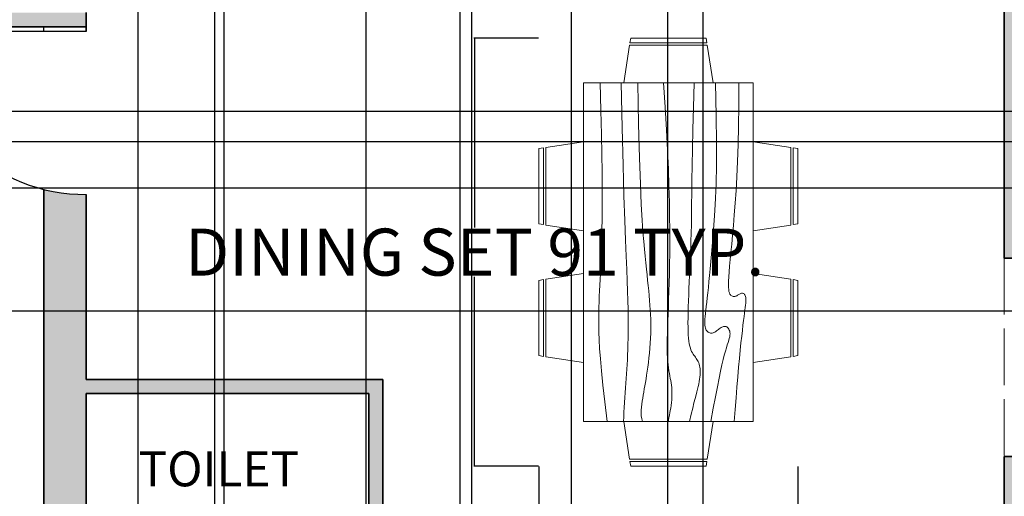
# Model space of a CAD drawing. Units: inches. Extents: x 300 to 1007, y 2 to 1069.
# Tile 3 of 12: x 557 to 766, y 170 to 271. Entities that reach past the tile are written whole.
import ezdxf

# ---------------------------------------------------------------- set-up
doc = ezdxf.new("R2010")
doc.units = ezdxf.units.IN
doc.header["$MEASUREMENT"] = 0
doc.linetypes.add('ACAD_ISO02W100', pattern=[15, 12, -3])
for name, color, linetype, lineweight in [('A-ANNO-DIMS', 2, 'Continuous', 18), ('A-AREA-IDEN', 7, 'Continuous', 18), ('A-DOOR', 3, 'Continuous', 25), ('A-FURN', 8, 'Continuous', 18), ('A-WALL', 7, 'Continuous', 35), ('A-WALL-OVHD', 8, 'ACAD_ISO02W100', 18)]:
    doc.layers.add(name, color=color, linetype=linetype, lineweight=lineweight)
doc.layers.add('A-WALL-PATT', color=9, linetype='Continuous', lineweight=9, true_color=0xc7c8ca)
doc.styles.get("Standard").update_dxf_attribs({"font": 'arial.ttf'})
doc.dimstyles.get("Standard").update_dxf_attribs({"dimtxt": 10, "dimasz": 0.18, "dimexe": 0.18, "dimexo": 0.0625, "dimgap": 0.09, "dimtad": 0, "dimtih": 1, "dimtoh": 1, "dimdec": 0, "dimzin": 0, "dimdsep": 46, "dimlunit": 3, "dimtxsty": 'Standard', "dimcen": 0.09, "dimadec": 0, "dimazin": 0, "dimtfac": 1, "dimtdec": 0, "dimtofl": 0, "dimtmove": 0, "dimatfit": 3, "dimfxl": 1, "dimtolj": 1, "dimtzin": 0, "dimarcsym": 0})

# ---------------------------------------------------------------- blocks, each defined once
blk = doc.blocks.new('Dining Set - 36 x 72 in.')
for p, q in [((-22, 27.5), (-22.1562, 26.50042)), ((-22, 27.5), (-6, 27.5)), ((-5.8437, 26.49966), (-6, 27.5)), ((6, 27.5), (5.8438, 26.50042)), ((6, 27.5), (22, 27.5)), ((22.1563, 26.49966), (22, 27.5)), ((-22.2343, 26.00059), (-23.4847, 17.99762)), ((-22.2304, 26), (-5.7608, 26)), ((-5.8416, 26.5), (-22.1534, 26.5)), ((-4.5152, 17.99762), (-5.7655, 25.99926)), ((5.7657, 26.00059), (4.5153, 17.99762)), ((5.7696, 26), (22.2392, 26)), ((22.1584, 26.5), (5.8466, 26.5)), ((23.4848, 17.99762), (22.2345, 25.99926)), ((36, 18), (-36, 18)), ((-36, 18), (-36, -18)), ((36, -18), (36, 18)), ((-44.0006, 8.23428), (-35.9976, 9.48474)), ((44.0006, 8.23428), (35.9976, 9.48474)), ((-45.5, 8), (-44.5004, 8.15617)), ((-45.5, 8), (-45.5, -8)), ((-44.5, -8.15843), (-44.5, 8.15338)), ((-44, 8.23041), (-44, -8.23915)), ((44, 8.23041), (44, -8.23915)), ((44.5, -8.15843), (44.5, 8.15338)), ((45.5, 8), (44.5005, 8.15617)), ((45.5, 8), (45.5, -8)), ((-44.4997, -8.15631), (-45.5, -8)), ((-35.9976, -9.48476), (-43.9993, -8.2345)), ((35.9976, -9.48476), (43.9993, -8.2345)), ((44.4997, -8.15631), (45.5, -8)), ((-36, -18), (36, -18)), ((-22.2343, -26.0006), (-23.4847, -17.99762)), ((-4.5152, -17.99762), (-5.7655, -25.99928)), ((5.7657, -26.0006), (4.5153, -17.99762)), ((23.4848, -17.99762), (22.2345, -25.99928)), ((-22.2304, -26), (-5.7608, -26)), ((-22, -27.5), (-22.1562, -26.50044)), ((-5.8416, -26.5), (-22.1534, -26.5)), ((-5.8437, -26.49967), (-6, -27.5)), ((5.7696, -26), (22.2392, -26)), ((6, -27.5), (5.8438, -26.50044)), ((22.1584, -26.5), (5.8466, -26.5)), ((22.1563, -26.49967), (22, -27.5)), ((-22, -27.5), (-6, -27.5)), ((6, -27.5), (22, -27.5))]:
    blk.add_line(p, q)
for points in [[(-36, 15), (-31.1772, 14.97754), (-26.8079, 14.91406), (-22.8538, 14.81543), (-19.276, 14.6875), (-16.0362, 14.53613), (-13.0957, 14.36718), (-10.4159, 14.18652), (-7.9583, 14), (-5.6904, 13.81315), (-3.6035, 13.63021), (-1.6954, 13.45508), (0.0365, 13.29166), (1.5945, 13.14388), (2.9811, 13.01562), (4.1988, 12.9108), (5.25, 12.83333), (6.1393, 12.78613), (6.8802, 12.76823), (7.4883, 12.77767), (7.9792, 12.8125), (8.3685, 12.87077), (8.6719, 12.95052), (8.9049, 13.0498), (9.0833, 13.16666), (9.2205, 13.29899), (9.3216, 13.44401), (9.3895, 13.59879), (9.4271, 13.76041), (9.4373, 13.92594), (9.4232, 14.09245), (9.3875, 14.257), (9.3333, 14.41666), (9.2638, 14.56917), (9.1836, 14.71484), (9.0975, 14.85465), (9.0104, 14.98958), (8.9272, 15.1206), (8.8529, 15.2487), (8.7922, 15.37483), (8.75, 15.5), (8.7305, 15.62467), (8.7344, 15.74739), (8.7617, 15.86621), (8.8125, 15.97916), (8.8867, 16.08431), (8.9844, 16.17968), (9.1055, 16.26334), (9.25, 16.33333), (9.4189, 16.38802), (9.6172, 16.42708), (9.8506, 16.45052), (10.125, 16.45833), (10.4463, 16.45052), (10.8203, 16.42708), (11.2529, 16.38802), (11.75, 16.33333), (12.3184, 16.26318), (12.9694, 16.17838), (13.7151, 16.07991), (14.5677, 15.96875), (15.5395, 15.84586), (16.6426, 15.71224), (17.8893, 15.56884), (19.2917, 15.41666), (20.859, 15.25667), (22.5879, 15.08984), (24.4721, 14.91715), (26.5052, 14.73958), (28.6809, 14.5581), (30.9929, 14.3737), (33.4347, 14.18733), (36, 14)], [(-36, 10), (-28.9766, 10.14274), (-23.1725, 10.20442), (-18.4241, 10.19775), (-14.5677, 10.13541), (-11.4399, 10.03011), (-8.877, 9.89453), (-6.7154, 9.74137), (-4.7917, 9.58333), (-2.9698, 9.43082), (-1.2246, 9.28515), (0.4415, 9.14534), (2.026, 9.01041), (3.5266, 8.87939), (4.9408, 8.7513), (6.266, 8.62516), (7.5, 8.5), (8.6411, 8.37549), (9.6914, 8.2539), (10.6538, 8.13818), (11.5312, 8.03125), (12.3267, 7.93603), (13.043, 7.85547), (13.6831, 7.79248), (14.25, 7.75), (14.7471, 7.7303), (15.1797, 7.73307), (15.5537, 7.75732), (15.875, 7.80208), (16.1494, 7.86637), (16.3828, 7.94922), (16.5811, 8.04964), (16.75, 8.16666), (16.8944, 8.29915), (17.0143, 8.44531), (17.1089, 8.60319), (17.1771, 8.77083), (17.218, 8.94629), (17.2305, 9.1276), (17.2137, 9.31282), (17.1667, 9.5), (17.0895, 9.6875), (16.987, 9.875), (16.8649, 10.0625), (16.7292, 10.25), (16.5856, 10.4375), (16.4401, 10.625), (16.2985, 10.8125), (16.1667, 11), (16.05, 11.18733), (15.9518, 11.3737), (15.8752, 11.5581), (15.8229, 11.73958), (15.798, 11.91715), (15.8034, 12.08984), (15.842, 12.25667), (15.9167, 12.41666), (16.0295, 12.56836), (16.1784, 12.70833), (16.3605, 12.83268), (16.5729, 12.9375), (16.8127, 13.01888), (17.0768, 13.07291), (17.3625, 13.0957), (17.6667, 13.08333), (17.9894, 13.03312), (18.3418, 12.94726), (18.7382, 12.82918), (19.1927, 12.68229), (19.7195, 12.51001), (20.3327, 12.31575), (21.0465, 12.10294), (21.875, 11.875), (22.8357, 11.63354), (23.959, 11.37304), (25.2786, 11.08618), (26.8282, 10.76562), (28.6414, 10.40405), (30.752, 9.99414), (33.1936, 9.52856), (36, 9)], [(-36, 5.5), (-30.7157, 5.3348), (-26.069, 5.20963), (-21.9946, 5.11767), (-18.4271, 5.05208), (-15.3009, 5.00602), (-12.5508, 4.97265), (-10.1112, 4.94515), (-7.9167, 4.91666), (-5.909, 4.88167), (-4.0586, 4.83984), (-2.3429, 4.79215), (-0.7396, 4.73958), (0.7739, 4.6831), (2.22, 4.6237), (3.6213, 4.56233), (5, 4.5), (6.373, 4.43782), (7.7344, 4.3776), (9.0723, 4.32129), (10.375, 4.27083), (11.6309, 4.22819), (12.8281, 4.19531), (13.9551, 4.17415), (15, 4.16666), (15.954, 4.17448), (16.819, 4.19791), (17.6001, 4.23698), (18.3021, 4.29166), (18.9299, 4.36198), (19.4883, 4.44791), (19.9823, 4.54948), (20.4167, 4.66666), (20.7969, 4.79899), (21.1302, 4.94401), (21.4245, 5.09879), (21.6875, 5.26041), (21.9271, 5.42594), (22.1511, 5.59245), (22.3672, 5.757), (22.5834, 5.91666), (22.8065, 6.06868), (23.0404, 6.21093), (23.2879, 6.34147), (23.5521, 6.45833), (23.8358, 6.55957), (24.142, 6.64323), (24.4735, 6.70735), (24.8334, 6.75), (25.2235, 6.76969), (25.642, 6.76692), (26.0858, 6.74267), (26.5521, 6.69791), (27.0379, 6.63362), (27.5404, 6.55078), (28.0565, 6.45036), (28.5834, 6.33333), (29.1242, 6.19987), (29.7071, 6.04687), (30.3661, 5.87044), (31.1354, 5.66666), (32.0493, 5.43164), (33.142, 5.16146), (34.4475, 4.85221), (36, 4.5)], [(-36, -1), (-30.7915, -0.6591), (-26.0195, -0.38216), (-21.6519, -0.16284), (-17.6563, 0.00521), (-14.0005, 0.12833), (-10.6523, 0.21289), (-7.5796, 0.26522), (-4.75, 0.29166), (-2.134, 0.29793), (0.2878, 0.28711), (2.5317, 0.26163), (4.6146, 0.22396), (6.5529, 0.17651), (8.3633, 0.12174), (10.0623, 0.06209), (11.6667, 0), (13.1899, -0.06201), (14.6341, -0.1211), (15.9982, -0.17432), (17.2813, -0.21875), (18.4823, -0.25147), (19.6003, -0.26953), (20.6343, -0.27002), (21.5834, -0.25), (22.4481, -0.20768), (23.2357, -0.14584), (23.9549, -0.06836), (24.6146, 0.02083), (25.2235, 0.11784), (25.7904, 0.21875), (26.3241, 0.31966), (26.8334, 0.41666), (27.3265, 0.50618), (27.8099, 0.58593), (28.2894, 0.65397), (28.7709, 0.70833), (29.2601, 0.74707), (29.763, 0.76823), (30.2855, 0.76985), (30.8334, 0.75), (31.4088, 0.70784), (31.9994, 0.64713), (32.589, 0.57275), (33.1615, 0.48958), (33.7008, 0.4025), (34.1908, 0.3164), (34.6153, 0.23616), (34.9584, 0.16666), (35.2099, 0.11165), (35.3848, 0.07031), (35.504, 0.04069), (35.5886, 0.02083), (35.6594, 0.00879), (35.7377, 0.0026), (35.8442, 0.00032), (36, 0)], [(-36, -6.5), (-27.1843, -6.31267), (-20.084, -6.1263), (-14.469, -5.9419), (-10.1094, -5.76042), (-6.7752, -5.58285), (-4.2363, -5.41016), (-2.2629, -5.24333), (-0.625, -5.08334), (0.8708, -4.93099), (2.2715, -4.78646), (3.5872, -4.64974), (4.8281, -4.52084), (6.0046, -4.39974), (7.127, -4.28646), (8.2053, -4.18099), (9.25, -4.08334), (10.2705, -3.99382), (11.2734, -3.91407), (12.2647, -3.84603), (13.25, -3.79167), (14.2354, -3.75293), (15.2266, -3.73177), (16.2295, -3.73015), (17.25, -3.75), (18.2912, -3.79248), (19.3451, -3.85547), (20.4009, -3.93604), (21.4479, -4.03125), (22.4754, -4.13819), (23.4727, -4.25391), (24.4289, -4.37549), (25.3334, -4.5), (26.1785, -4.62492), (26.9694, -4.74935), (27.7145, -4.87281), (28.4219, -4.99479), (29.1, -5.11483), (29.7572, -5.23242), (30.4016, -5.34709), (31.0417, -5.45834), (31.6837, -5.56437), (32.3262, -5.65821), (32.9658, -5.73153), (33.599, -5.77604), (34.2224, -5.78345), (34.8327, -5.74545), (35.4264, -5.65373), (36, -5.5)], [(-36, -10), (-26.4022, -9.81299), (-18.4675, -9.62891), (-11.9839, -9.45069), (-6.7396, -9.28125), (-2.5226, -9.12354), (0.8789, -8.98047), (3.6769, -8.85498), (6.0833, -8.75), (8.2767, -8.66765), (10.3021, -8.60677), (12.1712, -8.56543), (13.8958, -8.54167), (15.4876, -8.53353), (16.9583, -8.53907), (18.3197, -8.55632), (19.5834, -8.58334), (20.7616, -8.61841), (21.8685, -8.66081), (22.9188, -8.71004), (23.9271, -8.76563), (24.9081, -8.82707), (25.8763, -8.89388), (26.8465, -8.96558), (27.8334, -9.04167), (28.8474, -9.12118), (29.8828, -9.20117), (30.93, -9.27824), (31.9792, -9.34896), (33.0205, -9.40991), (34.0443, -9.45768), (35.0407, -9.48885), (36, -9.5)], [(-36, -14.5), (-30.0881, -14.33513), (-25.0332, -14.21224), (-20.7312, -14.12647), (-17.0781, -14.07292), (-13.97, -14.04671), (-11.3027, -14.04297), (-8.9724, -14.05681), (-6.875, -14.08334), (-4.9224, -14.11833), (-3.0905, -14.16016), (-1.3709, -14.20785), (0.2448, -14.26042), (1.7647, -14.3169), (3.1973, -14.3763), (4.5507, -14.43767), (5.8333, -14.5), (7.0554, -14.5621), (8.235, -14.62175), (9.3922, -14.67652), (10.5469, -14.72396), (11.7192, -14.76164), (12.929, -14.78711), (14.1965, -14.79794), (15.5417, -14.79167), (16.9933, -14.76424), (18.6152, -14.70508), (20.4804, -14.60197), (22.6615, -14.44271), (25.2312, -14.21509), (28.2624, -13.9069), (31.8277, -13.50594), (36, -13)]]:
    blk.add_lwpolyline(points)
blk = doc.blocks.new('DOOR-SINGLE-36')
for p, q in [((-1, 0), (-1, 36)), ((0, 0), (0, 36))]:
    blk.add_line(p, q)
blk.add_arc((0, 0.34), 35.66, 90, 180.5503)
blk = doc.blocks.new('*D53')
at = {"layer": 'A-ANNO-DIMS', "color": 0, "lineweight": -2, "transparency": 16777216}
for p, q in [((667.21, 266.96), (653.44, 266.96)), ((653.62, 266.78), (653.62, 226.72)), ((653.62, 176.14), (653.62, 216.2)), ((667.21, 175.96), (653.44, 175.96))]:
    blk.add_line(p, q, dxfattribs=at)
at = {"layer": 'A-ANNO-DIMS', "color": 0, "transparency": 16777216}
for points in [[(653.59, 266.78), (653.65, 266.78), (653.62, 266.96)], [(653.59, 176.14), (653.65, 176.14), (653.62, 175.96)]]:
    blk.add_solid(points, dxfattribs=at)
at = {"layer": 'Defpoints', "color": 0, "transparency": 16777216}
for p in [(667.27, 266.96), (653.62, 175.96), (667.27, 175.96)]:
    blk.add_point(p, dxfattribs=at)
at = {"layer": 'A-ANNO-DIMS', "color": 0, "transparency": 16777216, "insert": (653.62, 221.46), "char_height": 10, "attachment_point": 5}
blk.add_mtext('\\A1;DINING SET 91 TYP.', dxfattribs=at)
blk = doc.blocks.new('*D54')
at = {"layer": 'A-ANNO-DIMS', "color": 0, "lineweight": -2, "transparency": 16777216}
for p, q in [((667.27, 175.9), (667.27, 162.13)), ((722.27, 175.9), (722.27, 162.13)), ((667.45, 162.31), (670.34, 162.31)), ((722.09, 162.31), (719.2, 162.31))]:
    blk.add_line(p, q, dxfattribs=at)
at = {"layer": 'A-ANNO-DIMS', "color": 0, "transparency": 16777216}
for points in [[(667.45, 162.34), (667.45, 162.28), (667.27, 162.31)], [(722.09, 162.34), (722.09, 162.28), (722.27, 162.31)]]:
    blk.add_solid(points, dxfattribs=at)
at = {"layer": 'Defpoints', "color": 0, "transparency": 16777216}
for p in [(667.27, 175.96), (722.27, 175.96), (722.27, 162.31)]:
    blk.add_point(p, dxfattribs=at)
at = {"layer": 'A-ANNO-DIMS', "color": 0, "transparency": 16777216, "insert": (694.77, 162.31), "char_height": 10, "attachment_point": 5}
blk.add_mtext('\\A1;55 TYP.', dxfattribs=at)
blk = doc.blocks.new('*D87')
at = {"layer": 'A-ANNO-DIMS', "color": 0, "lineweight": -2, "transparency": 16777216}
for p, q in [((805.89, 251.38), (354.19, 251.38)), ((354.37, 251.2), (354.37, 248.43)), ((354.37, 235.26), (354.37, 238.03)), ((805.89, 235.08), (354.19, 235.08))]:
    blk.add_line(p, q, dxfattribs=at)
at = {"layer": 'A-ANNO-DIMS', "color": 0, "transparency": 16777216}
for points in [[(354.34, 251.2), (354.4, 251.2), (354.37, 251.38)], [(354.34, 235.26), (354.4, 235.26), (354.37, 235.08)]]:
    blk.add_solid(points, dxfattribs=at)
at = {"layer": 'Defpoints', "color": 0, "transparency": 16777216}
for p in [(805.95, 251.38), (354.37, 235.08), (805.95, 235.08)]:
    blk.add_point(p, dxfattribs=at)
at = {"layer": 'A-ANNO-DIMS', "color": 0, "transparency": 16777216, "insert": (354.37, 243.23), "char_height": 10, "attachment_point": 5}
blk.add_mtext('\\A1;16.3', dxfattribs=at)
blk = doc.blocks.new('*D89')
at = {"layer": 'A-ANNO-DIMS', "color": 0, "lineweight": -2, "transparency": 16777216}
for p, q in [((544.6, 83.45), (544.6, 1063.03)), ((544.78, 1062.85), (554.56, 1062.85)), ((598.25, 1062.85), (588.48, 1062.85)), ((598.43, 83.45), (598.43, 1063.03))]:
    blk.add_line(p, q, dxfattribs=at)
at = {"layer": 'A-ANNO-DIMS', "color": 0, "transparency": 16777216}
for points in [[(544.78, 1062.88), (544.78, 1062.82), (544.6, 1062.85)], [(598.25, 1062.88), (598.25, 1062.82), (598.43, 1062.85)]]:
    blk.add_solid(points, dxfattribs=at)
at = {"layer": 'Defpoints', "color": 0, "transparency": 16777216}
for p in [(598.43, 1062.85), (544.6, 83.38), (598.43, 83.38)]:
    blk.add_point(p, dxfattribs=at)
at = {"layer": 'A-ANNO-DIMS', "color": 0, "transparency": 16777216, "insert": (571.52, 1062.85), "char_height": 10, "attachment_point": 5}
blk.add_mtext('\\A1;53.83', dxfattribs=at)
blk = doc.blocks.new('*D90')
at = {"layer": 'A-ANNO-DIMS', "color": 0, "lineweight": -2, "transparency": 16777216}
for p, q in [((429.18, 209), (974.48, 209)), ((974.3, 208.82), (974.3, 151.39)), ((974.3, 83.56), (974.3, 141)), ((429.18, 83.38), (974.48, 83.38))]:
    blk.add_line(p, q, dxfattribs=at)
at = {"layer": 'A-ANNO-DIMS', "color": 0, "transparency": 16777216}
for points in [[(974.27, 208.82), (974.33, 208.82), (974.3, 209)], [(974.27, 83.56), (974.33, 83.56), (974.3, 83.38)]]:
    blk.add_solid(points, dxfattribs=at)
at = {"layer": 'Defpoints', "color": 0, "transparency": 16777216}
for p in [(429.12, 209), (974.3, 209), (429.12, 83.38)]:
    blk.add_point(p, dxfattribs=at)
at = {"layer": 'A-ANNO-DIMS', "color": 0, "transparency": 16777216, "insert": (974.3, 146.19), "char_height": 10, "attachment_point": 5}
blk.add_mtext('\\A1;125.61', dxfattribs=at)
blk = doc.blocks.new('*D91')
at = {"layer": 'A-ANNO-DIMS', "color": 0, "lineweight": -2, "transparency": 16777216}
for p, q in [((429.18, 325.09), (974.48, 325.09)), ((974.3, 324.91), (974.3, 290.23)), ((974.3, 245.16), (974.3, 279.84)), ((429.18, 244.98), (974.48, 244.98))]:
    blk.add_line(p, q, dxfattribs=at)
at = {"layer": 'A-ANNO-DIMS', "color": 0, "transparency": 16777216}
for points in [[(974.27, 324.91), (974.33, 324.91), (974.3, 325.09)], [(974.27, 245.16), (974.33, 245.16), (974.3, 244.98)]]:
    blk.add_solid(points, dxfattribs=at)
at = {"layer": 'Defpoints', "color": 0, "transparency": 16777216}
for p in [(429.12, 325.09), (974.3, 325.09), (429.12, 244.98)]:
    blk.add_point(p, dxfattribs=at)
at = {"layer": 'A-ANNO-DIMS', "color": 0, "transparency": 16777216, "insert": (974.3, 285.04), "char_height": 10, "attachment_point": 5}
blk.add_mtext('\\A1;80.11', dxfattribs=at)
blk = doc.blocks.new('*D102')
at = {"layer": 'A-ANNO-DIMS', "color": 0, "lineweight": -2, "transparency": 16777216}
for p, q in [((600.34, 609.38), (600.34, 8.45)), ((652.99, 609.38), (652.99, 8.45)), ((600.52, 8.63), (609.71, 8.63)), ((652.81, 8.63), (643.62, 8.63))]:
    blk.add_line(p, q, dxfattribs=at)
at = {"layer": 'A-ANNO-DIMS', "color": 0, "transparency": 16777216}
for points in [[(600.52, 8.66), (600.52, 8.6), (600.34, 8.63)], [(652.81, 8.66), (652.81, 8.6), (652.99, 8.63)]]:
    blk.add_solid(points, dxfattribs=at)
at = {"layer": 'Defpoints', "color": 0, "transparency": 16777216}
for p in [(600.34, 609.45), (652.99, 609.45), (652.99, 8.63)]:
    blk.add_point(p, dxfattribs=at)
at = {"layer": 'A-ANNO-DIMS', "color": 0, "transparency": 16777216, "insert": (626.66, 8.63), "char_height": 10, "attachment_point": 5}
blk.add_mtext('\\A1;52.66', dxfattribs=at)
blk = doc.blocks.new('*D103')
at = {"layer": 'A-ANNO-DIMS', "color": 0, "lineweight": -2, "transparency": 16777216}
for p, q in [((652.99, 609.38), (652.99, 8.45)), ((674.16, 609.38), (674.16, 8.45)), ((653.17, 8.63), (673.98, 8.63)), ((674.16, 8.63), (674.34, 8.63))]:
    blk.add_line(p, q, dxfattribs=at)
at = {"layer": 'A-ANNO-DIMS', "color": 0, "transparency": 16777216}
for points in [[(653.17, 8.66), (653.17, 8.6), (652.99, 8.63)], [(673.98, 8.66), (673.98, 8.6), (674.16, 8.63)]]:
    blk.add_solid(points, dxfattribs=at)
at = {"layer": 'Defpoints', "color": 0, "transparency": 16777216}
for p in [(652.99, 609.45), (674.16, 609.45), (674.16, 8.63)]:
    blk.add_point(p, dxfattribs=at)
at = {"layer": 'A-ANNO-DIMS', "color": 0, "transparency": 16777216, "insert": (695.25, 8.63), "char_height": 10, "attachment_point": 5}
blk.add_mtext('\\A1;21.164', dxfattribs=at)
blk = doc.blocks.new('*D104')
at = {"layer": 'A-ANNO-DIMS', "color": 0, "lineweight": -2, "transparency": 16777216}
for p, q in [((674.16, 609.38), (674.16, 8.45)), ((694.58, 609.38), (694.58, 8.45)), ((674.34, 8.63), (694.4, 8.63)), ((694.58, 8.63), (694.76, 8.63))]:
    blk.add_line(p, q, dxfattribs=at)
at = {"layer": 'A-ANNO-DIMS', "color": 0, "transparency": 16777216}
for points in [[(674.34, 8.66), (674.34, 8.6), (674.16, 8.63)], [(694.4, 8.66), (694.4, 8.6), (694.58, 8.63)]]:
    blk.add_solid(points, dxfattribs=at)
at = {"layer": 'Defpoints', "color": 0, "transparency": 16777216}
for p in [(674.16, 609.45), (694.58, 609.45), (694.58, 8.63)]:
    blk.add_point(p, dxfattribs=at)
at = {"layer": 'A-ANNO-DIMS', "color": 0, "transparency": 16777216, "insert": (711.75, 8.63), "char_height": 10, "attachment_point": 5}
blk.add_mtext('\\A1;20.42', dxfattribs=at)
blk = doc.blocks.new('*D106')
at = {"layer": 'A-ANNO-DIMS', "color": 0, "lineweight": -2, "transparency": 16777216}
for p, q in [((582.11, 990.38), (582.11, 8.45)), ((630.49, 990.38), (630.49, 8.45)), ((582.29, 8.63), (589.12, 8.63)), ((630.31, 8.63), (623.47, 8.63))]:
    blk.add_line(p, q, dxfattribs=at)
at = {"layer": 'A-ANNO-DIMS', "color": 0, "transparency": 16777216}
for points in [[(582.29, 8.66), (582.29, 8.6), (582.11, 8.63)], [(630.31, 8.66), (630.31, 8.6), (630.49, 8.63)]]:
    blk.add_solid(points, dxfattribs=at)
at = {"layer": 'Defpoints', "color": 0, "transparency": 16777216}
for p in [(582.11, 990.45), (630.49, 990.45), (630.49, 8.63)]:
    blk.add_point(p, dxfattribs=at)
at = {"layer": 'A-ANNO-DIMS', "color": 0, "transparency": 16777216, "insert": (606.3, 8.63), "char_height": 10, "attachment_point": 5}
blk.add_mtext('\\A1;48.38', dxfattribs=at)
blk = doc.blocks.new('*D107')
at = {"layer": 'A-ANNO-DIMS', "color": 0, "lineweight": -2, "transparency": 16777216}
for p, q in [((630.49, 990.38), (630.49, 8.45)), ((650.47, 990.38), (650.47, 8.45)), ((630.67, 8.63), (650.29, 8.63)), ((650.47, 8.63), (650.65, 8.63))]:
    blk.add_line(p, q, dxfattribs=at)
at = {"layer": 'A-ANNO-DIMS', "color": 0, "transparency": 16777216}
for points in [[(630.67, 8.66), (630.67, 8.6), (630.49, 8.63)], [(650.29, 8.66), (650.29, 8.6), (650.47, 8.63)]]:
    blk.add_solid(points, dxfattribs=at)
at = {"layer": 'Defpoints', "color": 0, "transparency": 16777216}
for p in [(630.49, 990.45), (650.47, 990.45), (650.47, 8.63)]:
    blk.add_point(p, dxfattribs=at)
at = {"layer": 'A-ANNO-DIMS', "color": 0, "transparency": 16777216, "insert": (667.15, 8.63), "char_height": 10, "attachment_point": 5}
blk.add_mtext('\\A1;19.98', dxfattribs=at)
blk = doc.blocks.new('*D108')
at = {"layer": 'A-ANNO-DIMS', "color": 0, "lineweight": -2, "transparency": 16777216}
for p, q in [((650.47, 990.38), (650.47, 8.45)), ((702.09, 990.38), (702.09, 8.45)), ((650.65, 8.63), (659.37, 8.63)), ((701.91, 8.63), (693.19, 8.63))]:
    blk.add_line(p, q, dxfattribs=at)
at = {"layer": 'A-ANNO-DIMS', "color": 0, "transparency": 16777216}
for points in [[(650.65, 8.66), (650.65, 8.6), (650.47, 8.63)], [(701.91, 8.66), (701.91, 8.6), (702.09, 8.63)]]:
    blk.add_solid(points, dxfattribs=at)
at = {"layer": 'Defpoints', "color": 0, "transparency": 16777216}
for p in [(650.47, 990.45), (702.09, 990.45), (702.09, 8.63)]:
    blk.add_point(p, dxfattribs=at)
at = {"layer": 'A-ANNO-DIMS', "color": 0, "transparency": 16777216, "insert": (676.28, 8.63), "char_height": 10, "attachment_point": 5}
blk.add_mtext('\\A1;51.62', dxfattribs=at)

msp = doc.modelspace()

# ---------------------------------------------------------------- hatches: boundary and pattern name
at = {"layer": 'A-WALL-PATT'}
h = msp.add_hatch(color=256, dxfattribs=at)
h.dxf.hatch_style = 1
h.paths.add_polyline_path([(546.104, 999.4468), (478.8267, 999.4468), (478.8267, 869.2798, -0.06322715), (487.8267, 868.1328), (487.8267, 990.4468), (546.104, 990.4468)])
h.paths.add_polyline_path([(630.4852, 999.4468), (582.106, 999.4468), (582.106, 990.4468), (613.8267, 990.4468), (613.8267, 867.4468), (622.8267, 867.4468), (622.8267, 990.4468), (630.4852, 990.4468)])
h.paths.add_polyline_path([(702.0883, 999.4468), (650.4653, 999.4468), (650.4653, 990.4468), (682.8267, 990.4468), (682.8267, 960.0824, -0.02530575), (685.8267, 960.0478), (685.8267, 990.4468), (702.0883, 990.4468)])
h.paths.add_polyline_path([(850.8267, 999.4468), (737.5888, 999.4468), (737.5888, 990.4468), (841.8267, 990.4468), (841.8267, 950.5685), (850.8267, 950.5685)])
h.paths.add_polyline_path([(685.8267, 930.4465), (682.8267, 930.4465), (682.8267, 888.4468), (682.8267, 867.4468), (685.8267, 867.4468), (697.4169, 867.4468), (697.4169, 870.4468), (685.8267, 870.4468), (685.8267, 888.4468)])
h.paths.add_polyline_path([(682.8267, 931.4465), (654.3436, 931.4465, 0.00843109), (654.3267, 930.4465), (682.8267, 930.4465)])
h.paths.add_polyline_path([(685.8267, 931.4465), (682.8267, 931.4465), (682.8267, 930.4465), (685.8267, 930.4465)])
h.paths.add_polyline_path([(682.8267, 888.4468), (622.8267, 888.4468), (622.8267, 885.4468), (682.8267, 885.4468)])
h.paths.add_polyline_path([(850.8267, 870.4468), (850.8267, 914.7851), (841.8267, 914.7851), (841.8267, 870.4468), (732.7101, 870.4468, -0.02120595), (732.8267, 867.4468), (779.8267, 867.4468), (779.8267, 749.4468), (782.8267, 749.4468), (788.8267, 749.4468), (788.8267, 861.4468), (841.8267, 861.4468), (841.8267, 749.4468), (850.8267, 749.4468)])
h.paths.add_polyline_path([(622.8267, 810.4468), (487.8267, 810.4468), (487.8267, 833.2626), (478.8267, 833.2626), (478.8267, 609.4468), (478.8267, 482.3847), (487.8267, 482.3847), (487.8267, 801.4468), (620.8267, 801.4468), (622.8267, 801.4468)])
h.paths.add_polyline_path([(680.8267, 729.4468), (620.8267, 729.4468), (620.8267, 765.8246, -0.02111352), (617.8267, 766.0562), (617.8267, 698.7303), (620.8267, 698.7303), (620.8267, 726.4468), (680.8267, 726.4468)])
h.paths.add_polyline_path([(620.8267, 668.8122, -0.02498293), (617.8267, 668.6448), (617.8267, 618.4468), (600.3357, 618.4468), (600.3357, 609.4468), (652.9929, 609.4468), (652.9929, 618.4468), (620.8267, 618.4468)])
h.paths.add_polyline_path([(552.3393, 618.4468), (487.8267, 618.4468), (487.8267, 609.4468), (552.3393, 609.4468)], flags=17)
h.paths.add_polyline_path([(694.5763, 618.4468), (683.8267, 618.4468), (683.8267, 726.4468), (683.8267, 749.4468), (680.8267, 749.4468), (680.8267, 740.4468), (680.8267, 726.4468), (680.8267, 618.4468), (674.1573, 618.4468), (674.1573, 609.4468), (680.8267, 609.4468), (694.5763, 609.4468)])
h.paths.add_polyline_path([(850.8267, 642.8902), (841.8267, 642.8902), (841.8267, 618.4468), (782.8267, 618.4468), (782.8267, 708.0513, -0.02308839), (779.8267, 707.9092), (779.8267, 618.4468), (730.1068, 618.4468), (730.1068, 609.4468), (779.8267, 609.4468), (841.8267, 609.4468), (841.8267, 482.3847), (850.8267, 482.3847)])
h.paths.add_polyline_path([(850.8267, 749.4468), (841.8267, 749.4468), (841.8267, 705.9119), (850.8267, 705.9119)])
h.paths.add_polyline_path([(841.8267, 749.4468), (782.8267, 749.4468), (779.8267, 749.4468), (761.9959, 749.4468), (761.9959, 740.4468), (779.8267, 740.4468), (812.3267, 740.4468), (841.8267, 740.4468)])
h.paths.add_polyline_path([(669.1457, 482.3847), (604.489, 482.3847), (604.489, 473.3847), (631.1217, 473.3847), (631.1217, 436.0244, -0.02504709), (634.1217, 436.1748), (634.1217, 436.4367), (634.1217, 473.3847), (669.1457, 473.3847)], flags=17)
h.paths.add_polyline_path([(580.5305, 482.3847), (571.1217, 482.3847), (541.0813, 482.3847), (541.0813, 473.3847), (562.1217, 473.3847), (562.1217, 326.3847), (571.1217, 326.3847), (571.1217, 362.3847), (631.1217, 362.3847), (631.1217, 326.3847), (706.9024, 326.3847, -0.02105388), (706.9999, 329.3847), (634.1217, 329.3847), (634.1217, 365.3847), (634.1217, 406.1748), (631.1217, 406.1748), (631.1217, 365.3847), (571.1217, 365.3847), (571.1217, 473.3847), (580.5305, 473.3847)])
h.paths.add_polyline_path([(493.4756, 482.3847), (420.1217, 482.3847), (420.1217, 445.3134), (429.1217, 445.3134), (429.1217, 473.3847), (493.4756, 473.3847)])
h.paths.add_polyline_path([(786.2236, 482.3847), (716.7793, 482.3847), (716.7793, 473.3847), (766.1217, 473.3847), (766.1217, 329.3847), (742.5583, 329.3847), (742.5583, 326.3847), (766.1217, 326.3847), (766.1217, 316.0647), (769.1217, 316.0647), (769.1217, 326.3847), (769.1217, 473.3847), (786.2236, 473.3847)])
h.paths.add_polyline_path([(910.1217, 482.3847), (822.7166, 482.3847), (822.7166, 473.3847), (901.1217, 473.3847), (901.1217, 402.5393), (910.1217, 402.5393)])
h.paths.add_polyline_path([(910.1217, 366.1034), (901.1217, 366.1034), (901.1217, 329.3847), (814.1217, 329.3847), (814.1217, 312.5176), (817.1217, 312.5176), (817.1217, 326.3847), (901.1217, 326.3847), (901.1217, 293.0319), (910.1217, 293.0319), (910.1217, 326.3847)])
h.paths.add_polyline_path([(910.1217, 268.9355), (901.1217, 268.9355), (901.1217, 254.3847), (817.1217, 254.3847), (817.1217, 290.5411, -0.03396715), (814.1217, 290.3847), (814.1217, 254.3847), (775.1217, 254.3847), (775.1217, 281.5164), (769.1217, 281.5164), (769.1217, 292.1577), (766.1217, 292.1577), (766.1217, 254.3847), (766.1217, 220.1938), (775.5079, 220.1938), (775.5079, 251.3847), (817.1217, 251.3847), (901.1217, 251.3847), (901.1217, 152.3847), (819.0246, 152.3847, -0.02493798), (818.9117, 149.3847), (901.1217, 149.3847), (901.1217, 92.3847), (901.1217, 83.3847), (874.3528, 83.3847), (874.3528, 74.3847), (910.1217, 74.3847), (910.1217, 92.3847), (910.1217, 149.3847)])
h.paths.add_polyline_path([(429.1217, 325.0924), (420.1217, 325.0924), (420.1217, 263.3847), (420.1217, 244.9834), (429.1217, 244.9834), (429.1217, 269.3847), (571.1217, 269.3847), (571.1217, 272.3847), (562.1217, 272.3847), (429.1217, 272.3847)])
h.paths.add_polyline_path([(429.1217, 208.998), (420.1217, 208.998), (420.1217, 74.3847), (496.7704, 74.3847), (496.7704, 83.3847), (429.1217, 83.3847)])
h.paths.add_polyline_path([(598.4322, 83.3847), (571.1217, 83.3847), (571.1217, 122.1171), (562.1217, 122.1171), (562.1217, 83.3847), (544.6031, 83.3847), (544.6031, 74.3847), (598.4322, 74.3847)])
h.paths.add_polyline_path([(797.0822, 83.3847), (769.1217, 83.3847), (769.1217, 149.3847), (788.9123, 149.3847), (788.9123, 152.3847), (769.1217, 152.3847), (769.1217, 178.0167), (766.1217, 178.0167), (766.1217, 152.3847), (735.3598, 152.3847), (735.3598, 143.3847), (766.1217, 143.3847), (766.1217, 83.3847), (634.1217, 83.3847), (634.1217, 143.3847), (659.7326, 143.3847), (659.7326, 152.3847), (634.1217, 152.3847), (634.1217, 194.3847), (571.1217, 194.3847), (571.1217, 233.7289, -0.06379947), (562.1217, 234.7942), (562.1217, 163.4485), (567.7403, 163.4485), (567.7403, 152.3847), (571.1217, 152.3847), (571.1217, 191.3847), (631.1217, 191.3847), (631.1217, 83.3847), (621.979, 83.3847), (621.979, 74.3847), (631.1217, 74.3847), (797.0822, 74.3847)])

# ---------------------------------------------------------------- linework, layer by layer
at = {"layer": 'A-DOOR'}
msp.add_line((562.1217, 268.3847), (562.1217, 269.3847), dxfattribs=at)
at = {"layer": 'A-WALL'}
for p, q in [((766.1217, 293.1577), (766.1217, 254.3847)), ((429.1217, 269.3847), (571.1217, 269.3847)), ((766.1217, 254.3847), (766.1217, 220.1938)), ((562.1217, 163.4485), (562.1217, 234.7942)), ((571.1217, 194.3847), (571.1217, 233.7289)), ((766.1217, 220.1938), (775.5079, 220.1938)), ((634.1217, 194.3847), (571.1217, 194.3847)), ((634.1217, 152.3847), (634.1217, 194.3847)), ((571.1217, 83.3847), (571.1217, 191.3847)), ((631.1217, 191.3847), (571.1217, 191.3847)), ((631.1217, 83.3847), (631.1217, 191.3847)), ((766.1217, 152.3847), (766.1217, 178.0167)), ((766.1217, 178.0167), (769.1217, 178.0167))]:
    msp.add_line(p, q, dxfattribs=at)
msp.add_lwpolyline([(571.1217, 268.3847), (571.1217, 272.3847)], dxfattribs=at)
at = {"layer": 'A-WALL-OVHD'}
msp.add_line((766.1217, 220.1938), (766.1217, 178.0167), dxfattribs=at)

# ---------------------------------------------------------------- block references
at = {"layer": 'A-DOOR', "rotation": 90.00000000000108}
msp.add_blockref('DOOR-SINGLE-36', (571.1217, 269.3847), dxfattribs=at)
at = {"layer": 'A-FURN', "rotation": 270}
msp.add_blockref('Dining Set - 36 x 72 in.', (694.7726, 221.4603), dxfattribs=at)

# ---------------------------------------------------------------- texts
at = {"layer": 'A-AREA-IDEN'}
msp.add_text('TOILET', height=7.43087, dxfattribs=at).set_placement((582.2535, 171.6655))

# ---------------------------------------------------------------- dimensions: what is measured, and where the dimension line sits
at = {"layer": 'A-ANNO-DIMS'}
for base, p1, p2, override, picture, middle in [((598.4322, 1062.8469), (544.6031, 83.3847), (598.4322, 83.3847), {"dimdec": 2, "dimlfac": 1, "dimrnd": 0, "dimzin": 0, "dimdsep": 46, "dimlunit": 2}, '*D89', (571.5176, 1062.8469)), ((630.4852, 8.6288), (582.106, 990.4468), (630.4852, 990.4468), {"dimdec": 2, "dimlfac": 1, "dimrnd": 0, "dimzin": 0, "dimdsep": 46, "dimlunit": 2}, '*D106', (606.2956, 8.6288)), ((650.4653, 8.6288), (630.4852, 990.4468), (650.4653, 990.4468), {"dimdec": 2, "dimlfac": 1, "dimrnd": 0, "dimzin": 0, "dimdsep": 46, "dimlunit": 2}, '*D107', (667.1473, 8.6288)), ((702.0883, 8.6288), (650.4653, 990.4468), (702.0883, 990.4468), {"dimdec": 2, "dimlfac": 1, "dimrnd": 0, "dimzin": 0, "dimdsep": 46, "dimlunit": 2}, '*D108', (676.2768, 8.6288)), ((652.9929, 8.6288), (600.3357, 609.4468), (652.9929, 609.4468), {"dimdec": 2, "dimlfac": 1, "dimrnd": 0, "dimzin": 0, "dimdsep": 46, "dimlunit": 2}, '*D102', (626.6643, 8.6288)), ((674.1573, 8.6288), (652.9929, 609.4468), (674.1573, 609.4468), {"dimdec": 3, "dimlfac": 1, "dimrnd": 0, "dimzin": 0, "dimdsep": 46, "dimlunit": 2}, '*D103', (695.2493, 8.6288)), ((694.5763, 8.6288), (674.1573, 609.4468), (694.5763, 609.4468), {"dimdec": 2, "dimlfac": 1, "dimrnd": 0, "dimzin": 0, "dimdsep": 46, "dimlunit": 2}, '*D104', (711.7529, 8.6288))]:
    dim = msp.add_linear_dim(base=base, p1=p1, p2=p2, dimstyle='Standard', override=override, dxfattribs=at)
    dim.commit()
    dim.dimension.update_dxf_attribs({"geometry": picture, "text_midpoint": middle})
for base, p1, p2, override, picture, middle in [((974.3023, 325.0924), (429.1217, 244.9834), (429.1217, 325.0924), {"dimdec": 2, "dimlfac": 1, "dimrnd": 0, "dimzin": 0, "dimdsep": 46, "dimlunit": 2}, '*D91', (974.3023, 285.0379)), ((354.3658, 235.0834), (805.95, 251.3847), (805.95, 235.0834), {"dimdec": 1, "dimlfac": 1, "dimrnd": 0, "dimzin": 0, "dimdsep": 46, "dimlunit": 2}, '*D87', (354.3658, 243.2341)), ((974.3023, 208.998), (429.1217, 83.3847), (429.1217, 208.998), {"dimdec": 2, "dimlfac": 1, "dimrnd": 0, "dimzin": 0, "dimdsep": 46, "dimlunit": 2}, '*D90', (974.3023, 146.1913))]:
    dim = msp.add_linear_dim(base=base, p1=p1, p2=p2, angle=90, dimstyle='Standard', override=override, dxfattribs=at)
    dim.commit()
    dim.dimension.update_dxf_attribs({"geometry": picture, "text_midpoint": middle})
dim = msp.add_linear_dim(base=(653.6226, 175.9603), p1=(667.2726, 266.9603), p2=(667.2726, 175.9603), angle=270, text='DINING SET <> TYP.', dimstyle='Standard', override={"dimdec": 0, "dimlfac": 1, "dimrnd": 0, "dimzin": 0, "dimdsep": 46, "dimlunit": 2}, dxfattribs=at)
dim.commit()
dim.dimension.update_dxf_attribs({"geometry": '*D53', "text_midpoint": (653.6226, 221.4603)})
dim = msp.add_linear_dim(base=(722.2726, 162.3103), p1=(667.2726, 175.9603), p2=(722.2726, 175.9603), text='<> TYP.', dimstyle='Standard', override={"dimdec": 0, "dimlfac": 1, "dimrnd": 0, "dimzin": 0, "dimdsep": 46, "dimlunit": 2}, dxfattribs=at)
dim.commit()
dim.dimension.update_dxf_attribs({"geometry": '*D54', "text_midpoint": (694.7726, 162.3103)})

doc.saveas('drawing.dxf')
